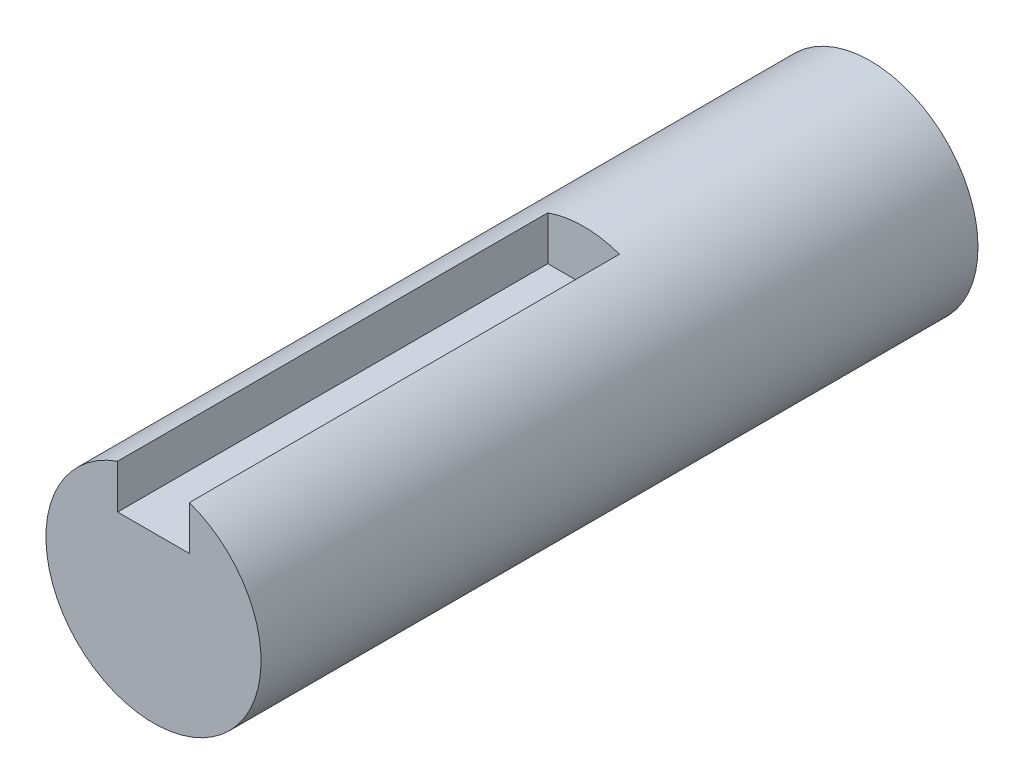
SolidWorks part; units mm, degrees
material "Plain Carbon Steel"
ref_plane "Front Plane" through (0, 0, 0) normal (0, 0, 1) x (1, 0, 0)
ref_plane "Top Plane" through (0, 0, 0) normal (0, 1, 0) x (1, 0, 0)
ref_plane "Right Plane" through (0, 0, 0) normal (1, 0, 0) x (0, 0, -1)
sketch "Shaft Profile Ø30" plane through (0, 0, 0) normal (0, 0, 1) x (1, 0, 0)
  circle A0 centre (0, 0) radius 15
  dimension "D1" = 30
extrude "Shaft Body Ø30x100" add sketch "Shaft Profile Ø30" along normal blind 100
sketch "Keyway Profile" plane through (0, 0, 100) normal (0, 0, 1) x (1, 0, 0)
  line L0 (0, 0) -> (0, 18.5574) construction
  line L2 (5, 15) -> (-5, 15)
  line L3 (5, 15) -> (5, 8)
  line L4 (5, 8) -> (-5, 8)
  line L5 (-5, 15) -> (-5, 8)
  dimension "D1" = 10
  dimension "D2" = 5
  dimension "D3" = 7
  dimension "D4" = 15
extrude "Keyway Cut 60mm" cut sketch "Keyway Profile" against normal blind 60
